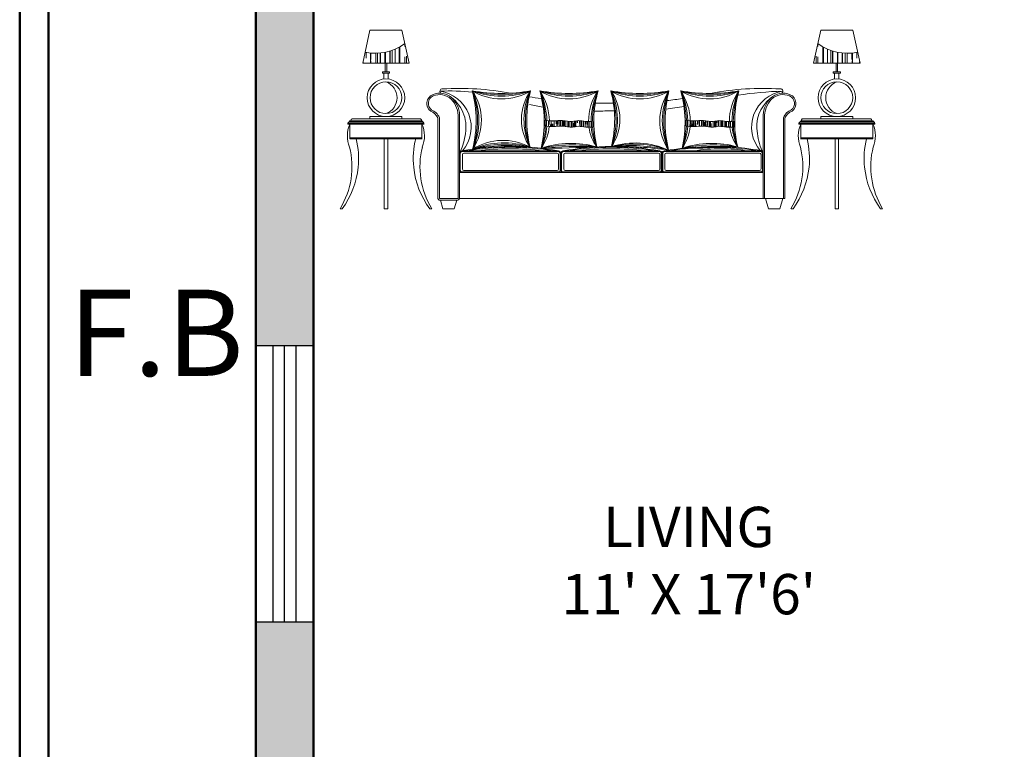
# Model space of a CAD drawing. Units: inches. Extents: x 1771 to 3025, y 319 to 889.
# Tile 18 of 35: x 2219 to 2390, y 621 to 747. Entities that reach past the tile are written whole.
import ezdxf

# ---------------------------------------------------------------- set-up
doc = ezdxf.new("R2010")
doc.units = ezdxf.units.IN
doc.header["$MEASUREMENT"] = 0
doc.set_wipeout_variables(frame=1)
for name, color, linetype, lineweight in [('A-AREA-IDEN', 241, 'Continuous', 25), ('A-FURN', 8, 'Continuous', 18), ('A-GLAZ', 40, 'Continuous', 25), ('A-WALL', 7, 'Continuous', 50), ('A-WALL-PATT', 254, 'Continuous', 13)]:
    doc.layers.add(name, color=color, linetype=linetype, lineweight=lineweight)
doc.styles.get("Standard").update_dxf_attribs({"font": 'arial.ttf'})

# ---------------------------------------------------------------- blocks, each defined once
blk = doc.blocks.new('A$C301F3DA3')
for p, q in [((156.7, 1006), (206.7, 1236)), ((206.7, 1236), (427.8, 1236)), ((477.8, 1006), (427.8, 1236)), ((3275.4, 1006), (3325.4, 1236)), ((3546.5, 1236), (3325.4, 1236)), ((3596.5, 1006), (3546.5, 1236)), ((344.5, 1006), (344.5, 1090.3)), ((347, 1006), (347, 1091.1)), ((359.5, 1006), (359.5, 1095.2)), ((380.5, 1006), (380.5, 1103.5)), ((409.5, 1006), (409.5, 1117.6)), ((411, 1006), (411, 1118.4)), ((414, 1006), (414, 1120.1)), ((447.5, 1121.4), (447.5, 1141.6)), ((3305.7, 1121.4), (3305.7, 1141.6)), ((3339.2, 1006), (3339.2, 1120.1)), ((3342.2, 1006), (3342.2, 1118.4)), ((3343.7, 1006), (3343.7, 1117.6)), ((3372.7, 1006), (3372.7, 1103.5)), ((3393.7, 1006), (3393.7, 1095.2)), ((3406.2, 1006), (3406.2, 1091.1)), ((3408.7, 1006), (3408.7, 1090.3)), ((179.5, 1041.4), (179.5, 1081.1)), ((209.5, 1006), (209.5, 1076.8)), ((211.5, 1060.9), (211.5, 1076.6)), ((211.5, 1006), (211.5, 1023.4)), ((213, 1031.4), (213, 1076.5)), ((246.5, 1006), (246.5, 1075.2)), ((259.5, 1006), (259.5, 1075.6)), ((278, 1006), (278, 1073.4)), ((280, 1006), (280, 1077.1)), ((309.5, 1006), (309.5, 1081.6)), ((313.5, 1006), (313.5, 1082.4)), ((447.5, 1006), (447.5, 1051.4)), ((459.5, 1006), (459.5, 1056.4)), ((3293.7, 1006), (3293.7, 1056.4)), ((3305.7, 1006), (3305.7, 1051.4)), ((3439.7, 1006), (3439.7, 1082.4)), ((3443.7, 1006), (3443.7, 1081.6)), ((3473.2, 1006), (3473.2, 1077.1)), ((3475.2, 1006), (3475.2, 1073.4)), ((3493.7, 1006), (3493.7, 1075.6)), ((3506.7, 1006), (3506.7, 1075.2)), ((3540.2, 1031.4), (3540.2, 1076.5)), ((3541.7, 1060.9), (3541.7, 1076.6)), ((3541.7, 1006), (3541.7, 1023.4)), ((3543.7, 1006), (3543.7, 1076.8)), ((3573.7, 1041.4), (3573.7, 1081.1)), ((156.7, 1006), (477.8, 1006)), ((159.5, 1006), (159.5, 1019)), ((312.2, 948), (312.2, 1006)), ((322.2, 948), (322.2, 1006)), ((322.2, 948), (322.2, 1006)), ((477.5, 1006), (477.5, 1007.2)), ((3596.5, 1006), (3275.4, 1006)), ((3275.7, 1006), (3275.7, 1007.2)), ((3431, 948), (3431, 1006)), ((3431, 948), (3431, 1006)), ((3441, 948), (3441, 1006)), ((3593.7, 1006), (3593.7, 1019)), ((292.2, 938), (292.2, 948)), ((342.2, 948), (292.2, 948)), ((342.2, 938), (292.2, 938)), ((302.2, 896.9), (302.2, 938)), ((332.2, 896.9), (332.2, 938)), ((342.2, 938), (342.2, 948)), ((3411, 938), (3411, 948)), ((3411, 948), (3461, 948)), ((3411, 938), (3461, 938)), ((3421, 896.9), (3421, 938)), ((3451, 896.9), (3451, 938)), ((3461, 938), (3461, 948)), ((557.5, 620.8), (82.9, 620.8)), ((206.3, 637.8), (428.1, 637.8)), ((206.3, 637.8), (206.3, 620.8)), ((428.1, 637.8), (428.1, 620.8)), ((3195.6, 620.8), (3670.3, 620.8)), ((3546.9, 637.8), (3325, 637.8)), ((3325, 637.8), (3325, 620.8)), ((3546.9, 637.8), (3546.9, 620.8)), ((53.7, 590.8), (53.7, 584.4)), ((67.1, 584.4), (67.1, 484)), ((565.7, 608.8), (75.3, 608.8)), ((557.5, 608.8), (82.9, 608.8)), ((3187.5, 608.8), (3677.9, 608.8)), ((3195.6, 608.8), (3670.3, 608.8)), ((3686.1, 584.4), (3686.1, 484)), ((3699.5, 590.8), (3699.5, 584.4)), ((305.2, 484), (305.2, 0)), ((329.2, 484), (329.2, 0)), ((3424, 484), (3424, 0)), ((3448, 484), (3448, 0)), ((0, 0), (14.7, 0)), ((329.2, 0), (305.2, 0)), ((3424, 0), (3448, 0)), ((3753.2, 0), (3738.4, 0))]:
    blk.add_line(p, q)
for centre, radius in [((317.2, 767.8), 130), ((3436, 767.8), 130), ((317.2, 767.8), 110), ((3436, 767.8), 110)]:
    blk.add_circle(centre, radius)
for centre, radius, start, end in [((243.2, 1422.6), 347.4, 258.38286, 306.14668), ((3510, 1422.6), 347.4, 233.85332, 281.61714), ((276.7, 767.8), 117.2, 290.217, 69.783), ((3476.5, 767.8), 117.2, 110.217, 249.783), ((86.1, 609.2), 12.1, 105.22692, 181.3736), ((551.7, 609.3), 12.5, 357.63421, 66.98041), ((3201.5, 609.3), 12.5, 113.01959, 182.36579), ((3667.1, 609.2), 12.1, 358.6264, 74.77308), ((250.8, 503.3), 200.8, 156.16528, 202.38219), ((63.8, 591), 10.1, 100.6467, 181.11305), ((74, 595.7), 13.1, 84.28738, 156.7847), ((3679.2, 595.7), 13.1, 23.2153, 95.71262), ((3502.4, 503.3), 200.8, 337.61781, 23.83472), ((3689.4, 591), 10.1, 358.88695, 79.3533), ((-428.9, 346.4), 557.3, 353.82498, 14.29835), ((1063.3, 346.4), 557.3, 165.70165, 186.17502), ((2689.9, 346.4), 557.3, 353.82498, 14.29835), ((4182.1, 346.4), 557.3, 165.70165, 186.17502), ((-472, 290.4), 554.2, 328.39652, 14.25331), ((4225.2, 290.4), 554.2, 165.74669, 211.60348), ((-467.1, 350.3), 595.7, 323.98153, 353.84466), ((4220.2, 350.3), 595.7, 186.15534, 216.01847)]:
    blk.add_arc(centre, radius, start, end)
blk.add_wipeout([(3041.8, 0), (2963.5, 0), (2943.5, 70), (826.6, 70), (824.2, 65.5), (819.2, 61.4), (815.3, 60), (806.8, 60), (789.7, 0), (711.4, 0), (694.3, 60), (685.4, 60), (681.9, 61.7), (678.1, 65.9), (676.6, 70), (676.6, 628.7), (667.5, 644), (650.9, 661.4), (635.1, 671.5), (625.4, 676.3), (610.1, 693.4), (602.5, 710.5), (600.1, 728.4), (604.2, 751.4), (623, 778.5), (639.5, 788.9), (669, 798), (689.6, 799.7), (696.6, 800), (691.2, 806.8), (690.2, 814.9), (693.8, 823.2), (701.1, 828), (705.9, 828.8), (865.5, 832), (984.1, 825.9), (1111.6, 811), (1170.7, 801.2), (1180.3, 799.4), (1231.4, 803.5), (1293.2, 811.6), (1317.6, 815.8), (1310.3, 786.3), (1307.6, 774.2), (1389.8, 761.2), (1393.6, 767.5), (1388.1, 790.9), (1381.5, 815.8), (1418.2, 809.7), (1480.9, 802.2), (1546.1, 798.2), (1588.9, 797.6), (1683.4, 802), (1730, 807.2), (1784.7, 815.8), (1774.6, 776.7), (1767.8, 744), (1769.2, 730.8), (1890.2, 730.7), (1884.7, 761.4), (1877, 795.8), (1871.7, 815.8), (1919.1, 808.2), (1966.4, 802.7), (2026, 798.6), (2073.3, 797.6), (2145.9, 799.9), (2221.5, 807.4), (2273.8, 815.4), (2267.3, 783.6), (2260.5, 748.2), (2369.1, 762), (2361.7, 794), (2355.9, 815.8), (2402.1, 808.4), (2442.8, 803.5), (2477.3, 800.5), (2535.4, 797.9), (2572.4, 797.9), (2610.4, 806.1), (2648.6, 812), (2670.2, 815.1), (2740.7, 823.3), (2819.6, 829.3), (2905.4, 832.2), (2981.5, 831.5), (3045.3, 828.6), (3053.9, 827.3), (3059.6, 822.9), (3062.8, 816.3), (3062.9, 810.1), (3060.6, 804.3), (3056.6, 800), (3070.6, 799.5), (3085.9, 797.7), (3105.1, 792.4), (3120.7, 785.3), (3134.4, 774.5), (3143.7, 762.3), (3150.7, 746.2), (3153, 725.9), (3150.1, 708.7), (3142.9, 693.1), (3133.2, 681), (3126.6, 675.3), (3114.9, 669.8), (3100.2, 659.6), (3082.1, 638.7), (3076.6, 628.7), (3076.6, 70), (3061.8, 70)])
for p, q in [((3056.6, 800), (3056.6, 799.5)), ((676.6, 70), (676.6, 628.7)), ((686.6, 70), (686.6, 630.8)), ((816.6, 70), (816.6, 647.2)), ((826.6, 70), (826.6, 627.7)), ((2926.6, 70), (2926.6, 647.2)), ((2936.6, 70), (2936.6, 647.2)), ((3066.6, 70), (3066.6, 630.8)), ((3076.6, 70), (3076.6, 628.7)), ((580.7, 590.8), (53.7, 590.8)), ((580.7, 584.4), (53.7, 584.4)), ((61.9, 600.9), (572.5, 600.9)), ((566.3, 584.4), (566.3, 484)), ((579.7, 590.8), (579.7, 584.4)), ((3172.5, 590.8), (3699.5, 590.8)), ((3172.5, 584.4), (3699.5, 584.4)), ((3173.5, 590.8), (3173.5, 584.4)), ((3691.3, 600.9), (3180.7, 600.9)), ((3186.9, 584.4), (3186.9, 484)), ((567.3, 490), (67.1, 490)), ((567.3, 484), (67.1, 484)), ((3185.9, 490), (3686.1, 490)), ((3185.9, 484), (3686.1, 484)), ((826.6, 400), (826.6, 265)), ((1511.6, 400), (841.6, 400)), ((1511.2, 395), (841.6, 395)), ((846.6, 275), (846.6, 375)), ((856.6, 385), (1501.6, 385)), ((1511.6, 375), (1511.6, 275)), ((1526.6, 265), (1526.6, 385)), ((1526.6, 265), (1526.6, 385)), ((1531.6, 265.4), (1531.6, 384.6)), ((1541.6, 400), (2211.6, 400)), ((1542, 395), (2211.2, 395)), ((1546.6, 275), (1546.6, 375)), ((1556.6, 385), (2201.6, 385)), ((2211.6, 375), (2211.6, 275)), ((2221.6, 384.6), (2221.6, 265.4)), ((2226.6, 265), (2226.6, 385)), ((2226.6, 385), (2226.6, 265)), ((2231.6, 265.4), (2231.6, 384.6)), ((2241.6, 400), (2911.6, 400)), ((2242, 395), (2911.2, 395)), ((2246.6, 275), (2246.6, 375)), ((2256.6, 385), (2901.6, 385)), ((2911.6, 375), (2911.6, 275)), ((2921.6, 384.6), (2921.6, 265.4)), ((1511.6, 250), (826.6, 250)), ((2926.6, 250), (826.6, 250)), ((841.6, 250), (1511.6, 250)), ((842, 255), (1511.6, 255)), ((1501.6, 265), (856.6, 265)), ((2211.6, 255), (1542, 255)), ((2201.6, 265), (1556.6, 265)), ((2911.2, 255), (2242, 255)), ((2901.6, 265), (2256.6, 265)), ((686.6, 70), (816.6, 70)), ((2926.6, 70), (826.6, 70)), ((2926.6, 70), (3076.6, 70)), ((3061.8, 70), (2943.5, 70)), ((2943.5, 70), (2963.5, 0)), ((3041.8, 0), (3061.8, 70)), ((633.4, 0), (618.7, 0)), ((685.4, 60), (815.3, 60)), ((711.4, 0), (694.3, 60)), ((789.7, 0), (711.4, 0)), ((806.8, 60), (789.7, 0)), ((2963.5, 0), (3041.8, 0)), ((3119.8, 0), (3134.5, 0))]:
    blk.add_line(p, q)
at = {"ltscale": 0.1}
for p, q in [((1414.4, 573.7), (1414.4, 606.7)), ((1418.8, 573), (1418.8, 612.1)), ((1420.6, 572.7), (1420.6, 580.7)), ((1427.8, 571.6), (1427.8, 610.7)), ((1440.6, 576.7), (1440.6, 609)), ((1441.2, 569.8), (1441.2, 608.9)), ((1445.4, 583.3), (1445.4, 608.4)), ((1454.6, 568.5), (1454.6, 582.7)), ((1460.6, 568.1), (1460.6, 607.2)), ((1468, 606.7), (1468, 607)), ((1468, 567.8), (1468, 586.7)), ((1472, 603.3), (1472, 606.9)), ((1472, 567.8), (1472, 588.3)), ((1480.6, 568.1), (1480.6, 588.7)), ((1481.4, 568.1), (1481.4, 607.3)), ((1494.8, 586.7), (1494.8, 608.3)), ((1498.6, 569.5), (1498.6, 608.3)), ((1500.6, 569.7), (1500.6, 608.8)), ((1508.2, 582.7), (1508.2, 609.5)), ((1520.6, 571.3), (1520.6, 610.4)), ((1521.6, 571.4), (1521.6, 610.5)), ((1525.2, 571.5), (1525.2, 610.6)), ((1535, 571.6), (1535, 610.7)), ((1540.6, 571.3), (1540.6, 610.4)), ((1548.4, 570.6), (1548.4, 609.6)), ((1551.8, 570.1), (1551.8, 609.2)), ((1560.6, 568.8), (1560.6, 607.9)), ((1561.8, 568.6), (1561.8, 607.7)), ((1575.2, 566.4), (1575.2, 605.5)), ((1578.4, 565.9), (1578.4, 605)), ((1580.6, 565.6), (1580.6, 604.7)), ((1588.6, 564.6), (1588.6, 603.7)), ((1600.6, 564), (1600.6, 603.1)), ((1602, 564), (1602, 590.7)), ((1605, 568.3), (1605, 603.3)), ((1615.4, 565.2), (1615.4, 594.7)), ((1620.6, 566.1), (1620.6, 600.7)), ((1628.8, 567.7), (1628.8, 606.9)), ((1631.6, 588.3), (1631.6, 607.4)), ((1631.6, 568.2), (1631.6, 581.7)), ((1640.6, 596.7), (1640.6, 608.8)), ((1642.2, 594.7), (1642.2, 609)), ((1655.6, 590.7), (1655.6, 609.3)), ((1655.6, 570.2), (1655.6, 570.7)), ((1658.2, 608.3), (1658.2, 609.1)), ((1658.2, 570), (1658.2, 601.7)), ((1660.6, 569.8), (1660.6, 608.9)), ((1669, 568.8), (1669, 607.9)), ((1680.6, 566.9), (1680.6, 606)), ((1682.4, 570.7), (1682.4, 605.7)), ((1684.8, 566.2), (1684.8, 605.3)), ((1695.8, 566.7), (1695.8, 603.7)), ((1700.6, 584.7), (1700.6, 603.2)), ((1700.6, 564.1), (1700.6, 564.7)), ((1709.2, 563.6), (1709.2, 602.7)), ((1711.4, 581.7), (1711.4, 602.7)), ((1711.4, 563.6), (1711.4, 566.7)), ((1720.6, 563.7), (1720.6, 602.8)), ((1722.6, 563.7), (1722.6, 602.9)), ((1736, 564.6), (1736, 603.8)), ((1738, 601.7), (1738, 603.9)), ((1738, 564.8), (1738, 586.7)), ((1740.6, 565), (1740.6, 604.2)), ((1749.4, 565.9), (1749.4, 598.7)), ((2392.6, 573.1), (2392.6, 610.7)), ((2400.6, 571.9), (2400.6, 610.9)), ((2403, 571.5), (2403, 610.6)), ((2406, 571.1), (2406, 610.1)), ((2419.4, 569.4), (2419.4, 582.7)), ((2420.6, 569.2), (2420.6, 608.3)), ((2429.6, 583.5), (2429.6, 607.5)), ((2429.6, 568.4), (2429.6, 576.9)), ((2432.8, 606.7), (2432.8, 607.3)), ((2432.8, 568.2), (2432.8, 586.7)), ((2440.6, 567.9), (2440.6, 607)), ((2446.2, 567.8), (2446.2, 606.9)), ((2456.2, 603.5), (2456.2, 607.3)), ((2456.2, 568.1), (2456.2, 596.9)), ((2459.6, 586.7), (2459.6, 607.5)), ((2460.6, 568.4), (2460.6, 592.7)), ((2473, 582.7), (2473, 608.6)), ((2480.6, 588.7), (2480.6, 609.3)), ((2482.8, 570.4), (2482.8, 609.5)), ((2486.4, 570.7), (2486.4, 609.8)), ((2499.8, 571.5), (2499.8, 610.6)), ((2500.6, 571.5), (2500.6, 610.7)), ((2509.4, 576.9), (2509.4, 610.7)), ((2513.2, 571.4), (2513.2, 610.5)), ((2520.6, 570.8), (2520.6, 600.7)), ((2526.6, 570.1), (2526.6, 609.1)), ((2536, 596.9), (2536, 607.7)), ((2536, 568.6), (2536, 581.9)), ((2540, 568), (2540, 607)), ((2540.6, 576.7), (2540.6, 606.9)), ((2553.4, 565.8), (2553.4, 604.9)), ((2560.6, 564.9), (2560.6, 604)), ((2562.6, 564.7), (2562.6, 601.9)), ((2566.8, 564.3), (2566.8, 590.7)), ((2580.2, 564.2), (2580.2, 594.7)), ((2580.6, 564.2), (2580.6, 603.3)), ((2589.2, 565.2), (2589.2, 604.3)), ((2593.6, 565.9), (2593.6, 605.1)), ((2600.6, 567.2), (2600.6, 606.4)), ((2607, 594.7), (2607, 607.6)), ((2615.8, 569.8), (2615.8, 608.9)), ((2620.4, 590.7), (2620.4, 609.3)), ((2620.4, 570.2), (2620.4, 570.7)), ((2620.6, 570.2), (2620.6, 609.3)), ((2633.8, 570), (2633.8, 609)), ((2640.6, 569.2), (2640.6, 608.3)), ((2642.4, 569), (2642.4, 608)), ((2647.2, 570.7), (2647.2, 607.3)), ((2660.6, 566), (2660.6, 605.1)), ((2660.6, 566.7), (2660.6, 605.1)), ((2669, 564.8), (2669, 603.8)), ((2674, 564.2), (2674, 603.3)), ((2680.6, 563.8), (2680.6, 568.7)), ((2687.4, 563.6), (2687.4, 602.7)), ((2695.6, 581.9), (2695.6, 602.8)), ((2695.6, 563.7), (2695.6, 575.3)), ((2700.6, 564.7), (2700.6, 603.1)), ((2700.8, 563.9), (2700.8, 603.1)), ((2714.2, 565), (2714.2, 598.7)), ((2720.6, 565.6), (2720.6, 604.8)), ((2722.2, 601.9), (2722.2, 604.9)), ((2722.2, 565.8), (2722.2, 595.3)), ((2727.6, 566.4), (2727.6, 602.7))]:
    blk.add_line(p, q, dxfattribs=at)
at = {"ltscale": 0.2}
for p, q in [((831.6, 384.6), (831.6, 265.4)), ((1521.6, 265.4), (1521.6, 384.6))]:
    blk.add_line(p, q, dxfattribs=at)
for centre, radius, start, end in [((705.9, 812.9), 15.9, 82.92998, 233.99863), ((826.9, -1080.6), 1912.9, 79.35353, 93.56712), ((2926.5, -1083.7), 1916.1, 86.44665, 100.89711), ((3047.3, 812.9), 15.9, 306.00137, 97.07002), ((666.4, 728.4), 66.3, 113.9424, 233.11156), ((666.4, 728.4), 56.3, 113.9424, 233.11156), ((689.6, 677.8), 121.9, 45.5351, 114.26403), ((689.6, 677.8), 111.9, 45.5351, 114.26403), ((647.8, 638.7), 169.2, 356.50689, 44.75015), ((647.8, 638.7), 179.2, 356.50689, 44.75015), ((118.5, 608.8), 822.4, 346.1538, 14.5736), ((1116, 1923.3), 1125.7, 259.68325, 280.31675), ((2062.3, 614.6), 771.4, 164.88081, 194.22903), ((1820.4, 3753.3), 3022.9, 260.23295, 261.81056), ((611.7, 598.3), 800, 346.95646, 15.77378), ((1583.1, 1923.3), 1125.7, 259.68325, 280.31675), ((2517.6, 605.2), 762.6, 163.96966, 193.48898), ((2073.3, 1923.3), 1125.7, 259.68325, 280.31675), ((1147.1, 613.7), 752.3, 345.86352, 15.58525), ((3098.6, 604.6), 850.3, 165.62179, 193.5679), ((1932.8, 3753.3), 3022.9, 276.22345, 278.29852), ((2556.6, 1923.4), 1125.7, 259.73156, 280.36506), ((1586.1, 598.3), 800, 346.95646, 15.77378), ((3493.3, 605.3), 763.9, 163.98353, 193.47734), ((3105.4, 638.7), 179.2, 135.24985, 176.50689), ((3105.4, 638.7), 169.2, 135.24985, 183.49311), ((3063.6, 677.8), 121.9, 65.73597, 134.4649), ((3063.6, 677.8), 111.9, 65.73597, 134.4649), ((3086.8, 728.4), 56.3, 306.88844, 66.0576), ((3086.8, 728.4), 66.3, 306.88844, 66.0576), ((593.4, 589.7), 101.9, 23.83547, 68.81673), ((1820.4, 3753.3), 3022.9, 269.03014, 271.06523), ((1932.8, 3753.3), 3022.9, 268.93477, 269.19298), ((3159.8, 589.7), 101.9, 112.01062, 156.16453), ((593.4, 589.7), 91.9, 24.95202, 68.81673), ((3159.8, 589.7), 91.9, 111.18327, 155.04798), ((561.8, 599.3), 9.8, 9.61841, 76.53695), ((382.6, 503.3), 200.8, 337.61781, 23.83472), ((562.8, 585.5), 17.7, 17.55797, 60.68227), ((3370.5, 503.3), 200.8, 156.16528, 202.38219), ((3190.4, 585.5), 17.7, 119.31773, 162.44203), ((3191.3, 599.3), 9.8, 103.46305, 170.38159), ((1106.4, 290.4), 554.2, 165.74669, 211.60348), ((1176.6, -1455.4), 1885.4, 79.76537, 100.23463), ((1150.7, -658.8), 1096, 81.40397, 102.31547), ((1256.5, 13610.3), 13193.2, 270.58435, 272.25734), ((1876.6, -1455.4), 1885.4, 79.76537, 100.23463), ((1933.3, -1830.3), 2260.9, 81.38364, 91.43687), ((2584.1, -1540.1), 1970.1, 79.98833, 100.01167), ((2230.8, 13610.3), 13193.2, 270.58435, 272.25734), ((2646.8, 290.4), 554.2, 328.39652, 14.25331), ((844.1, 382.5), 17.7, 98.1301, 171.8699), ((844.1, 382.5), 12.7, 101.3731, 171.8699), ((856.6, 375), 10, 90, 180), ((1501.6, 375), 10, 0, 90), ((1509.1, 382.5), 12.7, 9.60357, 81.8699), ((1509.1, 382.5), 17.7, 8.1301, 81.8699), ((1544.1, 382.5), 17.7, 98.1301, 171.8699), ((1544.1, 382.5), 12.7, 99.60357, 170.39643), ((1556.6, 375), 10, 90, 180), ((2201.6, 375), 10, 0, 90), ((2209.1, 382.5), 12.7, 9.60357, 81.8699), ((2209.1, 382.5), 17.7, 8.1301, 81.8699), ((2244.1, 382.5), 17.7, 98.1301, 171.8699), ((2244.1, 382.5), 12.7, 98.1301, 170.39643), ((2256.6, 375), 10, 90, 180), ((2901.6, 375), 10, 0, 90), ((2909.1, 382.5), 12.7, 9.60357, 80.39643), ((2909.1, 382.5), 17.7, 8.1301, 81.8699), ((1101.5, 350.3), 595.7, 186.15534, 216.01847), ((856.6, 275), 10, 180, 270), ((1501.6, 275), 10, 270, 0), ((1556.6, 275), 10, 180, 270), ((2201.6, 275), 10, 270, 0), ((2256.6, 275), 10, 180, 270), ((2901.6, 275), 10, 270, 0), ((2651.7, 350.3), 595.7, 323.98153, 353.84466), ((844.1, 267.5), 17.7, 188.1301, 261.8699), ((844.1, 267.5), 12.7, 189.60357, 260.39643), ((1509.1, 267.5), 12.7, 278.1301, 351.8699), ((1509.1, 267.5), 17.7, 278.1301, 351.8699), ((1544.1, 267.5), 17.7, 188.1301, 261.8699), ((1544.1, 267.5), 12.7, 188.1301, 261.8699), ((2209.1, 267.5), 12.7, 278.1301, 350.39643), ((2209.1, 267.5), 17.7, 278.1301, 351.8699), ((2244.1, 267.5), 17.7, 188.1301, 261.8699), ((2244.1, 267.5), 12.7, 189.60357, 261.8699), ((2909.1, 267.5), 12.7, 278.1301, 350.39643), ((2909.1, 267.5), 17.7, 278.1301, 351.8699), ((689.4, 72.4), 13, 190.46913, 252.22973), ((812.4, 74.7), 15, 281.33001, 341.83756)]:
    blk.add_arc(centre, radius, start, end)
for centre, radius, start, end in [((760.4, -701.1), 1515.6, 84.07641, 92.659), ((655.5, 564.2), 251.1, 319.40416, 82.09148), ((615.4, 566.9), 255.3, 349.39262, 57.21951), ((478.9, 611.1), 481.1, 335.55638, 25.17102), ((347.1, 610.3), 603.3, 340.81637, 19.91104), ((617, 612), 360.5, 326.31194, 34.41547), ((1116, 1147.7), 388.4, 238.72737, 301.27263), ((1116, 1532.7), 744.8, 254.29016, 285.61296), ((1116.1, 1337.7), 559.4, 249.04787, 290.9906), ((1594, 618.2), 339.8, 144.44675, 214.66309), ((1723.9, 617.2), 452.3, 153.95498, 205.15486), ((1847.8, 616.2), 566.5, 159.37514, 199.7347), ((757.4, 589.8), 663.8, 1.89953, 19.9071), ((904.2, 593.4), 526.6, 1.83653, 24.977), ((1057.3, 597.5), 390.8, 1.55805, 33.94797), ((1583.1, 1147.7), 388.4, 238.72737, 301.27263), ((1583.2, 1532.7), 744.8, 254.29016, 285.61296), ((1583.2, 1337.7), 559.4, 249.04787, 290.9906), ((2089.5, 604.3), 371, 145.24271, 180.23552), ((2233.6, 600.8), 497.7, 154.4139, 179.66501), ((2371.5, 597.7), 626, 159.61394, 179.36153), ((2073.3, 1147.7), 388.4, 238.72737, 301.27263), ((2073.4, 1532.7), 744.8, 254.29016, 285.61296), ((1604, 619.4), 332, 325.19263, 36.25614), ((1356.4, 616.3), 552.6, 340.29034, 21.15843), ((1477.2, 617.8), 441.4, 334.80604, 26.64273), ((2073.4, 1337.7), 559.4, 249.04787, 290.9906), ((2583.5, 608.3), 371.9, 146.08399, 213.1057), ((2726, 607.2), 497, 155.19256, 203.99713), ((2862.3, 606.3), 623.6, 160.37041, 198.81928), ((2557.2, 1147.9), 388.4, 238.77569, 301.32093), ((1731.8, 589.8), 663.8, 1.89953, 19.9071), ((1878.6, 593.4), 526.6, 1.83653, 24.977), ((2031.7, 597.5), 390.8, 1.55805, 33.94797), ((2556.9, 1532.9), 744.8, 254.33859, 285.66141), ((2557.2, 1337.9), 559.4, 249.09653, 291.03924), ((3065, 604.3), 372, 145.29362, 180.23636), ((3209.5, 600.8), 499.2, 154.45299, 179.66602), ((3347.8, 597.7), 627.9, 159.64574, 179.36278), ((3116.2, -1577.3), 2390.8, 91.27111, 98.78687), ((3097.7, 564.2), 251.1, 97.90852, 220.59584), ((3129.1, 568.5), 247.1, 128.48308, 191.34035), ((1756.4, 2902), 2227.1, 258.42921, 260.84468), ((1995, 2902), 2227.1, 276.64183, 279.91471), ((1756.4, 2902), 2227.1, 270.09381, 273.07097), ((1995, 2902), 2227.1, 266.92903, 267.47072), ((902.9, 592.1), 518.2, 340.3477, 357.85991), ((1016.3, 594.9), 414.5, 334.69408, 356.73006), ((1135.5, 598), 312.7, 324.80426, 354.71594), ((2016.9, 603.5), 298.4, 187.6695, 216.19187), ((2130.5, 600.8), 394.6, 185.24411, 206.08232), ((2238.4, 598.3), 492.9, 183.79515, 200.29326), ((1877.3, 592.1), 518.2, 340.3477, 357.85991), ((1990.7, 594.9), 414.5, 334.69408, 356.73006), ((2109.9, 598), 312.7, 324.80426, 354.71594), ((2991.3, 603.5), 298.4, 187.6695, 216.19187), ((3104.9, 600.8), 394.6, 185.24411, 206.08232), ((3212.8, 598.3), 492.9, 183.79515, 200.29326), ((468.9, 563.6), 399.8, 334.99578, 353.7174), ((3284.3, 563.6), 399.8, 186.2826, 206.53978), ((1176.6, -1429.1), 1854.1, 80.58034, 99.41966), ((1126.7, 81.6), 391.4, 61.31825, 122.4012), ((1138.5, -278.6), 725.3, 76.04293, 107.78495), ((1132.5, -88.7), 544.9, 70.60179, 113.1041), ((1176.6, -1342.3), 1757.3, 82.5085, 97.4915), ((1599, -199.4), 651.3, 74.21866, 108.62302), ((1646.2, -2030.8), 2461.8, 87.00101, 95.95019), ((1608.6, -583.8), 1025.1, 80.66015, 102.16113), ((1876.6, -1429.1), 1854.1, 80.58034, 99.41966), ((1876.6, -1429.1), 1844.1, 82.68708, 97.31292), ((2041.7, -102.7), 557.6, 65.60138, 107.21913), ((2031.9, -256.9), 704.2, 70.15873, 102.74025), ((2004.4, -699.8), 1137, 76.44399, 96.45498), ((2584.1, -1521.2), 1946.2, 80.80656, 99.19344), ((2573.4, -199.4), 651.3, 74.21866, 108.62302), ((2620.6, -2030.8), 2461.8, 87.00101, 95.95019), ((2583, -583.8), 1025.1, 80.66015, 102.16113), ((2634.1, -753.4), 1168.4, 80.80901, 99.19099)]:
    blk.add_arc(centre, radius, start, end, dxfattribs=at)
for points in [[(1411.2, 613.3), (1432, 609.9), (1474.4, 603.1), (1540.1, 616.4), (1597.7, 597.2), (1650.5, 614.1), (1699.8, 599.6), (1736.2, 603.6), (1755.3, 605.7)], [(2385.5, 613.3), (2406.4, 609.9), (2448.8, 603.1), (2514.5, 616.4), (2572, 597.2), (2624.9, 614.1), (2674.2, 599.6), (2710.6, 603.6), (2729.6, 605.7)], [(1411.5, 574.2), (1432.4, 570.8), (1474.8, 564), (1540.5, 577.3), (1598, 558.1), (1650.9, 575), (1700.2, 560.5), (1736.6, 564.5), (1755.6, 566.6)], [(2385.9, 574.2), (2406.8, 570.8), (2449.2, 564), (2514.8, 577.3), (2572.4, 558.1), (2625.2, 575), (2674.5, 560.5), (2711, 564.5), (2730, 566.6)]]:
    blk.add_open_spline(points, degree=3, knots=[0, 0, 0, 0, 62.941123, 128.023226, 196.918691, 236.354413, 288.676993, 345.703861, 345.703861, 345.703861, 345.703861])
blk = doc.blocks.new('WIN-48')
for p, q in [((0, 0), (0, 10)), ((48, 0), (48, 10)), ((0, 7), (48, 7)), ((0, 5), (48, 5)), ((0, 3), (48, 3))]:
    blk.add_line(p, q)

msp = doc.modelspace()

# ---------------------------------------------------------------- hatches: boundary and pattern name
at = {"layer": 'A-WALL-PATT'}
h = msp.add_hatch(color=256, dxfattribs=at)
h.dxf.hatch_style = 1
h.paths.add_polyline_path([(2407.16, 878.63), (2429.21, 878.63), (2429.21, 888.63), (2379.16, 888.63), (2379.16, 878.63), (2402.16, 878.63), (2402.16, 830.63), (2407.16, 830.63)])
h.paths.add_polyline_path([(2520.11, 888.63), (2477.21, 888.63), (2477.21, 878.63), (2498.16, 878.63), (2498.16, 794.63), (2402.16, 794.63), (2402.16, 758.63), (2402.16, 664.63), (2407.16, 664.63), (2407.16, 712), (2407.16, 789.63), (2515.16, 789.63), (2515.16, 794.63), (2503.16, 794.63), (2503.16, 878.63), (2520.11, 878.63)])
h.paths.add_polyline_path([(2561.16, 888.63), (2538.11, 888.63), (2538.11, 878.63), (2551.16, 878.63), (2551.16, 789.63), (2551.16, 768.61), (2561.16, 768.61)])
h.paths.add_polyline_path([(2561.16, 720.61), (2551.16, 720.61), (2551.16, 669.63), (2443.16, 669.63), (2443.16, 664.63), (2462.16, 664.63), (2462.16, 652.63), (2467.16, 652.63), (2467.16, 664.63), (2551.16, 664.63), (2551.16, 649.17), (2561.16, 649.17)])
h.paths.add_polyline_path([(2561.16, 631.17), (2551.16, 631.17), (2551.16, 616.63), (2462.16, 616.63), (2443.16, 616.63), (2443.16, 611.63), (2551.16, 611.63), (2551.16, 581.11), (2561.16, 581.11)])
h.paths.add_polyline_path([(2561.16, 533.11), (2551.16, 533.11), (2551.16, 479.63), (2407.16, 479.63), (2407.16, 616.63), (2397.16, 616.63), (2397.16, 543.63), (2306.16, 543.63), (2306.16, 533.63), (2397.16, 533.63), (2397.16, 469.63), (2551.16, 469.63), (2551.16, 452.76), (2561.16, 452.76)])
h.paths.add_polyline_path([(2561.16, 404.76), (2551.16, 404.76), (2551.16, 393.63), (2397.16, 393.63), (2397.16, 383.63), (2561.16, 383.63)])
h.paths.add_polyline_path([(2270.16, 642.58), (2260.16, 642.58), (2260.16, 533.63), (2270.16, 533.63)])
h.paths.add_polyline_path([(2270.16, 753.63), (2366.16, 753.63), (2366.16, 758.63), (2270.16, 758.63), (2270.16, 842.59, -0.008336), (2268.86, 842.63), (2260.16, 842.63), (2260.16, 690.58), (2270.16, 690.58)])
h.paths.add_polyline_path([(2331.16, 888.63), (2260.16, 888.63), (2260.16, 878.63), (2331.16, 878.63)])

# ---------------------------------------------------------------- linework, layer by layer
at = {"layer": 'A-WALL'}
for p, q in [((2219.16, 888.63), (2219.16, 533.63)), ((2224.16, 878.63), (2224.16, 533.63)), ((2260.16, 842.63), (2260.16, 533.63)), ((2270.16, 753.63), (2270.16, 533.63))]:
    msp.add_line(p, q, dxfattribs=at)

# ---------------------------------------------------------------- block references
at = {"layer": 'A-GLAZ', "rotation": 90.00000000000072}
msp.add_blockref('WIN-48', (2270.16, 642.58), dxfattribs=at)

# ---------------------------------------------------------------- texts
at = {"layer": 'A-AREA-IDEN', "attachment_point": 1}
for s, insert, char_height in [('\\pxqc;F.B', (2200.13, 700.35), 15), ("\\pxqc;LIVING \\P11' X 17'6'", (2292.62, 662.63), 7)]:
    msp.add_mtext_dynamic_manual_height_columns(s, width=85.4611, gutter_width=1, heights=[0], dxfattribs=dict(at, insert=insert, char_height=char_height))

# ---------------------------------------------------------------- next in the draw order: block references
at = {"layer": 'A-FURN', "xscale": 0.0251055470835414, "yscale": 0.0251055470835414, "zscale": 0.0251055470835414}
msp.add_blockref('A$C301F3DA3', (2274.81, 714.39), dxfattribs=at)

doc.saveas('drawing.dxf')
